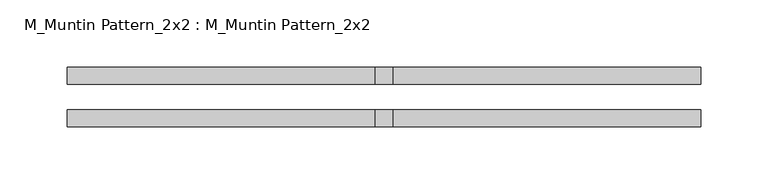
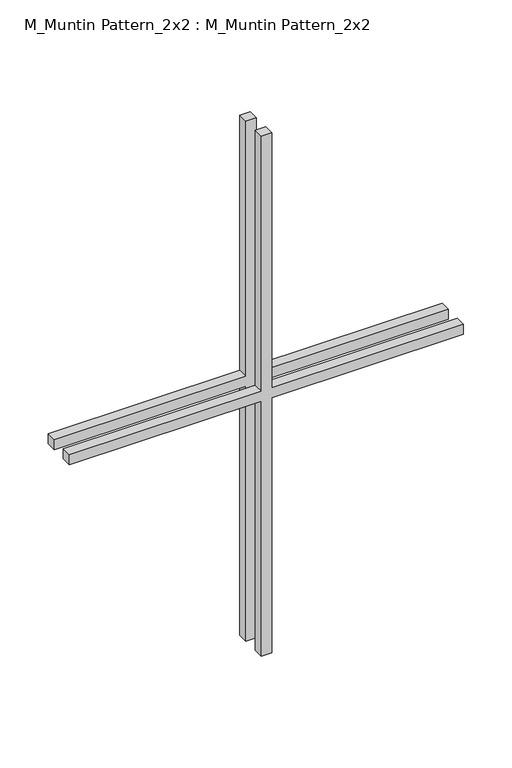
"""IFC4 building model written with IfcOpenShell, lengths in millimetres: proxy geometry, M_Muntin Pattern_2x2 : M_Muntin Pattern_2x2."""

from ifc_helpers import new_model, si_unit, frame, origin, place, context, project, spatial, polyline, outline, extrude, source, transform, mapped, element, save


def m_muntin_pattern_2x2_m_muntin_pattern_2x2_32a0f80e(model_context):
    return source(origin(), model_context, "Body", "SweptSolid", [
        extrude(outline(polyline([(336.5, -6.35), (336.5, -236.5375), (323.8, -236.5375), (323.8, -6.35), (0.0, -6.35), (0.0, 6.35), (323.8, 6.35), (323.8, 236.5375), (336.5, 236.5375), (336.5, 6.35), (660.3, 6.35), (660.3, -6.35), (336.5, -6.35)])), frame((0.0, -22.225, 0.0), z_axis=(0.0, 1.0, 0.0), x_axis=(0.0, 0.0, 1.0)), (0.0, 0.0, 1.0), 12.7),
        extrude(outline(polyline([(336.5, -6.35), (336.5, -236.5375), (323.8, -236.5375), (323.8, -6.35), (0.0, -6.35), (0.0, 6.35), (323.8, 6.35), (323.8, 236.5375), (336.5, 236.5375), (336.5, 6.35), (660.3, 6.35), (660.3, -6.35), (336.5, -6.35)])), frame((0.0, 9.525, 0.0), z_axis=(0.0, 1.0, 0.0), x_axis=(0.0, 0.0, 1.0)), (0.0, 0.0, 1.0), 12.7),
    ])


if __name__ == "__main__":
    model = new_model("IFC4")
    model_context = context("Model", 3, world=origin())
    ifc_project = project(units=[si_unit("LENGTHUNIT", "METRE", prefix="MILLI")], contexts=[model_context])
    site = spatial("IfcSite", under=ifc_project)
    building = spatial("IfcBuilding", under=site)
    placement = place(None, origin())
    m_muntin_pattern_2x2_m_muntin_pattern_2x2_shape = m_muntin_pattern_2x2_m_muntin_pattern_2x2_32a0f80e(model_context)
    element("IfcBuildingElementProxy", 1, Name="M_Muntin Pattern_2x2 : M_Muntin Pattern_2x2", ObjectType="M_Muntin Pattern_2x2 : M_Muntin Pattern_2x2", at=placement, inside=building, context=model_context, shape_type="MappedRepresentation", body=[
        mapped(m_muntin_pattern_2x2_m_muntin_pattern_2x2_shape, transform((0.0, 0.0, 0.0), x_axis=(1.0, 0.0, 0.0), y_axis=(0.0, 1.0, 0.0), z_axis=(0.0, 0.0, 1.0))),
    ])
    save(model, "model.ifc")

# Revit data of these elements
# Type "M_Muntin Pattern_2x2 : M_Muntin Pattern_2x2"
#   Width [instance default] = 3' - 11.24409"
#   Thickness = 0' - 0 1/2"
#   Height [instance default] = 3' - 11.24409"
#   Distance = 0' - 0 3/4"
#   Interior Material [instance default] = none
#   Exterior Material [instance default] = none
#   Default Elevation = 0
# Element 1 (IfcBuildingElementProxy, "M_Muntin Pattern_2x2 : M_Muntin Pattern_2x2")
#   Width = 1' - 6 5/8"
#   Height = 2' - 1.99606"
#   Interior Material = Wood - Stained
#   Exterior Material = Clad - White
#   Materials on its faces: "Clad - White", "Wood - Stained"
# Materials
#   "Clad - White": class "Wood", colour RGB 242 242 238, transparency 0, Cost = 0
#   "Wood - Stained": class "Wood", colour RGB 224 178 126, transparency 0, Cost = 0
